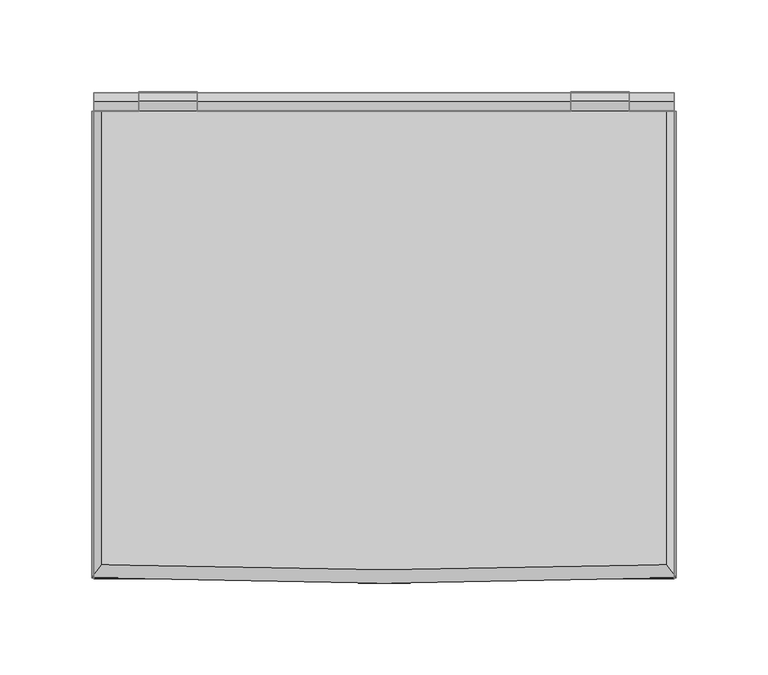
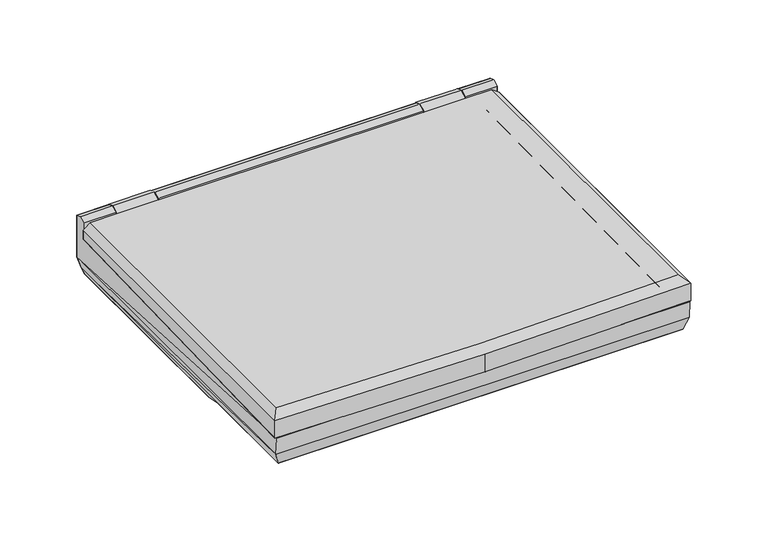
"""IFC4 building model written with IfcOpenShell, lengths in millimetres: proxy geometry."""

from ifc_helpers import new_model, si_unit, origin, place, context, project, spatial, triangles, source, transform, mapped, element, save


def entourage_4c8cfd20(model_context):
    return source(origin(), model_context, "Body", "Tessellation", [
        triangles([(-158.4296647, -167.5812681, 28.2218875), (-101.7496669, 97.7313983, 35.1332139), (-101.7496669, 97.7313983, 48.4910491), (-101.7496669, 92.7961799, 50.2665039), (-101.7496669, 87.9168539, 48.1837095), (-101.7496669, 87.9168539, 35.1332139), (-158.4296647, 87.9168539, 35.1332139), (-133.8221823, 97.7288549, 35.1332139), (-133.8221823, 97.7313983, 48.4910491), (-133.8221823, 92.7961799, 50.2665039), (-133.8221823, 87.9168539, 48.1837095), (-133.8221823, 87.9168539, 35.1332139), (158.4322081, -167.5812681, 28.2218875), (101.7496669, 97.7313983, 35.1332139), (101.7496669, 97.7313983, 48.4910491), (101.7496669, 92.7961799, 50.2665039), (101.7496669, 87.9168539, 48.1837095), (101.7496669, 87.9168539, 35.1332139), (85.2320795, -66.8399745, 31.8083601), (-144.8813274, -53.1646373, 31.9658404), (85.2320795, -53.1646373, 31.9658404), (-144.8813274, 60.6703247, 34.190875), (146.9209376, 74.3380406, 34.2924744), (146.9209376, -66.8399745, 31.8083601), (158.4322081, 87.9168539, 35.1332139), (133.8247257, 97.7313983, 35.1332139), (133.8247257, 97.7313983, 48.4910491), (133.8247257, 92.7961799, 50.2665039), (133.8247257, 87.9168539, 48.1837095), (133.8247257, 87.9168539, 35.1332139), (-142.7070869, 58.4935499, 29.3902845), (15.8851303, 74.3380406, 34.2924744), (19.0347234, 72.5752803, 29.491884), (15.8851303, 60.6703247, 34.190875), (19.0347234, 58.4935499, 29.3902845), (-155.2851437, -164.0506697, 4.7853507), (-155.2851437, -83.3296248, 4.869171), (-153.4715916, -69.0040502, 0.0), (-153.4715916, 95.8771965, 0.0), (155.2876871, -164.0506697, 4.7853507), (155.2851437, -83.3296248, 4.869171), (153.4715916, -69.0040502, 0.0), (153.4715916, 95.8771965, 0.0), (-155.2851437, 97.7313983, 4.869171), (-158.4296647, 97.7313983, 14.9046918), (-158.4296647, 97.7313983, 48.4910491), (155.2851437, 97.7313983, 4.869171), (158.4322081, 97.7313983, 14.9046918), (158.4322081, 97.7313983, 48.4910491), (-158.4296647, 92.7961799, 50.2665039), (-158.4296647, 87.9168539, 48.1837095), (158.4322081, 92.7961799, 50.2665039), (158.4322081, 87.9168539, 48.1837095), (-158.6201509, -166.809095, 14.9046918), (158.6201509, -166.809095, 14.9046918), (87.4063109, -64.9654568, 27.0992089), (-142.7070869, -51.2901242, 27.2541481), (87.4063109, -51.2901242, 27.2541481), (144.7467062, 72.5752803, 29.491884), (144.7467062, -64.9654568, 27.0992089), (141.2262725, -62.1181243, 32.971677), (90.9267446, -62.1181243, 32.971677), (-138.3738576, -48.4427871, 33.1266163), (90.9267446, -48.4427871, 33.1266163), (-138.3738576, 55.455713, 35.1128935), (141.2262725, 69.5374479, 35.2170342), (21.8820582, 55.455713, 35.1128935), (21.8820582, 69.5374479, 35.2170342), (0.0, 78.9883291, 38.7773751), (0.0, -148.3190173, 34.6998691), (-145.6915886, 78.9897371, 38.772488), (-145.6915886, -148.3190173, 34.6998691), (145.109929, 78.9897371, 38.772488), (145.109929, -148.3190173, 34.6998691), (0.0, 80.5417862, 35.3042041), (0.0, -149.5301715, 31.5516783), (-147.9064607, 80.5407416, 35.2986221), (-147.9064607, -149.5301715, 31.5516783), (147.3248011, 80.5407416, 35.2986221), (147.3248011, -149.5301715, 31.5516783), (0.0, -169.8360542, 28.0754711), (0.0, -169.7931244, 42.3380044), (-159.4431202, -167.0172945, 28.4001878), (-159.4431202, -166.9750733, 42.6651647), (159.4431202, -167.0172945, 28.4001878), (159.4431202, -166.9750733, 42.6651647), (0.0, -162.5080131, 46.5302948), (0.0, 87.4703786, 47.1442926), (-101.7496669, 98.2048796, 48.5682428), (-154.0176883, -159.6892353, 46.8550116), (-101.7496669, 87.4703786, 47.1442926), (-133.8221823, 98.2034989, 48.5546353), (-133.7332887, 87.4703786, 47.1442926), (-154.0176883, 87.4703786, 47.1442926), (-133.8221823, 93.2694705, 50.3265112), (-101.7496669, 93.2694705, 50.3265112), (-159.4431202, 87.4719228, 42.9645241), (101.7496669, 98.2048796, 48.5682428), (154.0176883, -159.6892353, 46.8550116), (101.7496669, 87.4703786, 47.1442926), (133.8221823, 98.2034989, 48.5546353), (133.7332887, 87.4703786, 47.1442926), (154.0176883, 87.4703786, 47.1442926), (133.8221823, 93.2694705, 50.3265112), (101.7496669, 93.2694705, 50.3265112), (159.4431202, 87.4719228, 42.9645241), (0.0, 87.4749477, 35.3976872), (-101.7496669, 98.2071505, 35.1985783), (-101.7496669, 87.4735397, 35.4025697), (-133.8221823, 98.2071505, 35.1985783), (101.7496669, 98.2071505, 35.1985783), (101.7496669, 87.4735397, 35.4025697), (133.8221823, 98.2071505, 35.1985783), (-133.7332887, 87.4735397, 35.4025697), (-159.4431202, 87.4732036, 35.3945465), (133.7332887, 87.4735397, 35.4025697), (159.4431202, 87.4732036, 35.3945465), (0.0, -167.5662254, 28.1582286), (-156.9437634, -164.7481562, 28.4853888), (-159.4431202, -69.7213121, 31.0754356), (0.0, -165.6878881, 31.2097138), (-155.5010462, -162.8722714, 31.5361724), (156.9437634, -164.7481562, 28.4853888), (159.4431202, -69.7213121, 31.0754356), (155.5010462, -162.8722714, 31.5361724)], [[19, 1, 13], [2, 6, 3], [3, 6, 4], [4, 6, 5], [12, 6, 8], [8, 6, 2], [11, 12, 10], [10, 12, 9], [9, 12, 8], [21, 20, 19], [20, 1, 19], [22, 6, 12], [1, 20, 7], [22, 12, 7], [23, 6, 32], [18, 6, 23], [19, 13, 24], [14, 15, 18], [15, 16, 18], [16, 17, 18], [30, 26, 18], [26, 14, 18], [29, 28, 30], [28, 27, 30], [27, 26, 30], [24, 25, 23], [23, 30, 18], [13, 25, 24], [23, 25, 30], [32, 6, 22], [22, 34, 32], [31, 33, 35], [37, 41, 36], [36, 41, 40], [42, 41, 38], [38, 41, 37], [39, 43, 38], [38, 43, 42], [44, 8, 2], [8, 44, 45], [45, 46, 9], [9, 8, 45], [44, 47, 39], [39, 47, 43], [2, 14, 47], [2, 47, 44], [3, 15, 14], [3, 14, 2], [47, 14, 26], [26, 48, 47], [48, 27, 49], [27, 48, 26], [50, 51, 11], [11, 10, 50], [5, 17, 16], [5, 16, 4], [52, 29, 53], [29, 52, 28], [46, 50, 10], [10, 9, 46], [4, 16, 15], [4, 15, 3], [49, 28, 52], [28, 49, 27], [13, 1, 55], [55, 1, 54], [55, 54, 40], [40, 54, 36], [55, 40, 41], [48, 52, 25], [52, 48, 49], [53, 25, 52], [41, 43, 47], [13, 48, 25], [55, 47, 48], [43, 41, 42], [48, 13, 55], [47, 55, 41], [51, 7, 12], [12, 11, 51], [6, 18, 17], [6, 17, 5], [53, 30, 25], [30, 53, 29], [54, 37, 36], [45, 7, 50], [50, 46, 45], [51, 50, 7], [37, 44, 39], [1, 7, 45], [54, 45, 44], [39, 38, 37], [45, 54, 1], [44, 37, 54], [57, 31, 22], [23, 32, 33], [33, 59, 23], [20, 21, 58], [58, 57, 20], [21, 19, 56], [56, 58, 21], [19, 24, 60], [60, 56, 19], [24, 23, 59], [59, 60, 24], [34, 22, 31], [31, 35, 34], [33, 32, 34], [34, 35, 33], [59, 35, 33], [20, 22, 7], [22, 20, 57], [67, 65, 63], [67, 63, 64], [64, 62, 61], [66, 64, 61], [31, 57, 63], [63, 65, 31], [35, 31, 65], [65, 67, 35], [57, 58, 64], [64, 63, 57], [58, 56, 62], [62, 64, 58], [56, 60, 61], [61, 62, 56], [60, 59, 66], [66, 61, 60], [66, 67, 64], [68, 66, 59], [59, 33, 68], [35, 67, 68], [68, 33, 35], [66, 68, 67], [69, 70, 72], [69, 72, 71], [69, 74, 70], [69, 73, 74], [76, 78, 72], [72, 70, 76], [77, 75, 69], [69, 71, 77], [78, 77, 71], [71, 72, 78], [76, 74, 80], [74, 76, 70], [79, 69, 75], [69, 79, 73], [80, 73, 79], [73, 80, 74], [81, 82, 84], [81, 84, 83], [81, 86, 82], [81, 85, 86], [82, 87, 90], [82, 90, 84], [87, 88, 91], [87, 91, 90], [90, 91, 93], [96, 89, 92], [96, 92, 95], [90, 93, 94], [97, 90, 94], [91, 95, 93], [91, 96, 95], [97, 84, 90], [82, 99, 87], [82, 86, 99], [87, 100, 88], [87, 99, 100], [99, 102, 100], [105, 101, 98], [105, 104, 101], [102, 99, 103], [106, 103, 99], [100, 102, 104], [100, 104, 105], [106, 99, 86], [89, 108, 110], [89, 110, 92], [96, 91, 89], [89, 91, 108], [108, 91, 109], [91, 88, 109], [109, 88, 107], [98, 113, 111], [98, 101, 113], [105, 98, 100], [98, 111, 100], [111, 112, 100], [100, 112, 88], [112, 107, 88], [93, 114, 115], [93, 115, 97], [95, 92, 93], [93, 92, 114], [114, 92, 110], [93, 97, 94], [102, 117, 116], [102, 106, 117], [104, 102, 101], [102, 116, 101], [116, 113, 101], [102, 103, 106], [108, 109, 114], [108, 114, 110], [81, 83, 119], [109, 107, 75], [75, 77, 109], [114, 109, 77], [120, 115, 77], [114, 77, 115], [119, 118, 81], [77, 78, 120], [119, 120, 122], [76, 121, 122], [76, 122, 78], [119, 122, 121], [119, 121, 118], [120, 78, 122], [83, 120, 119], [111, 116, 112], [111, 113, 116], [81, 123, 85], [112, 75, 107], [75, 112, 79], [116, 79, 112], [124, 79, 117], [117, 79, 116], [123, 81, 118], [79, 124, 80], [123, 125, 124], [76, 125, 121], [76, 80, 125], [123, 121, 125], [123, 118, 121], [124, 125, 80], [85, 123, 124], [117, 86, 124], [117, 106, 86], [124, 86, 85], [115, 120, 84], [115, 84, 97], [120, 83, 84]], closed=False),
    ])


if __name__ == "__main__":
    model = new_model("IFC4")
    model_context = context("Model", 3, world=origin())
    ifc_project = project(units=[si_unit("LENGTHUNIT", "METRE", prefix="MILLI")], contexts=[model_context])
    site = spatial("IfcSite", under=ifc_project)
    building = spatial("IfcBuilding", under=site)
    placement = place(None, origin())
    entourage_shape = entourage_4c8cfd20(model_context)
    element("IfcBuildingElementProxy", 1, Name="Entourage", at=placement, inside=building, context=model_context, shape_type="MappedRepresentation", body=[
        mapped(entourage_shape, transform((0.0, 0.0, 0.0), x_axis=(1.0, 0.0, 0.0), y_axis=(0.0, 1.0, 0.0), z_axis=(0.0, 0.0, 1.0))),
    ])
    save(model, "model.ifc")

# Revit data of these elements
# Type
#   built-in parameter 1005195 = "RPC-16-N04H-AQSP-D1N4-43SU-6GKQ-C3KU-1C"
#   Height = 0
